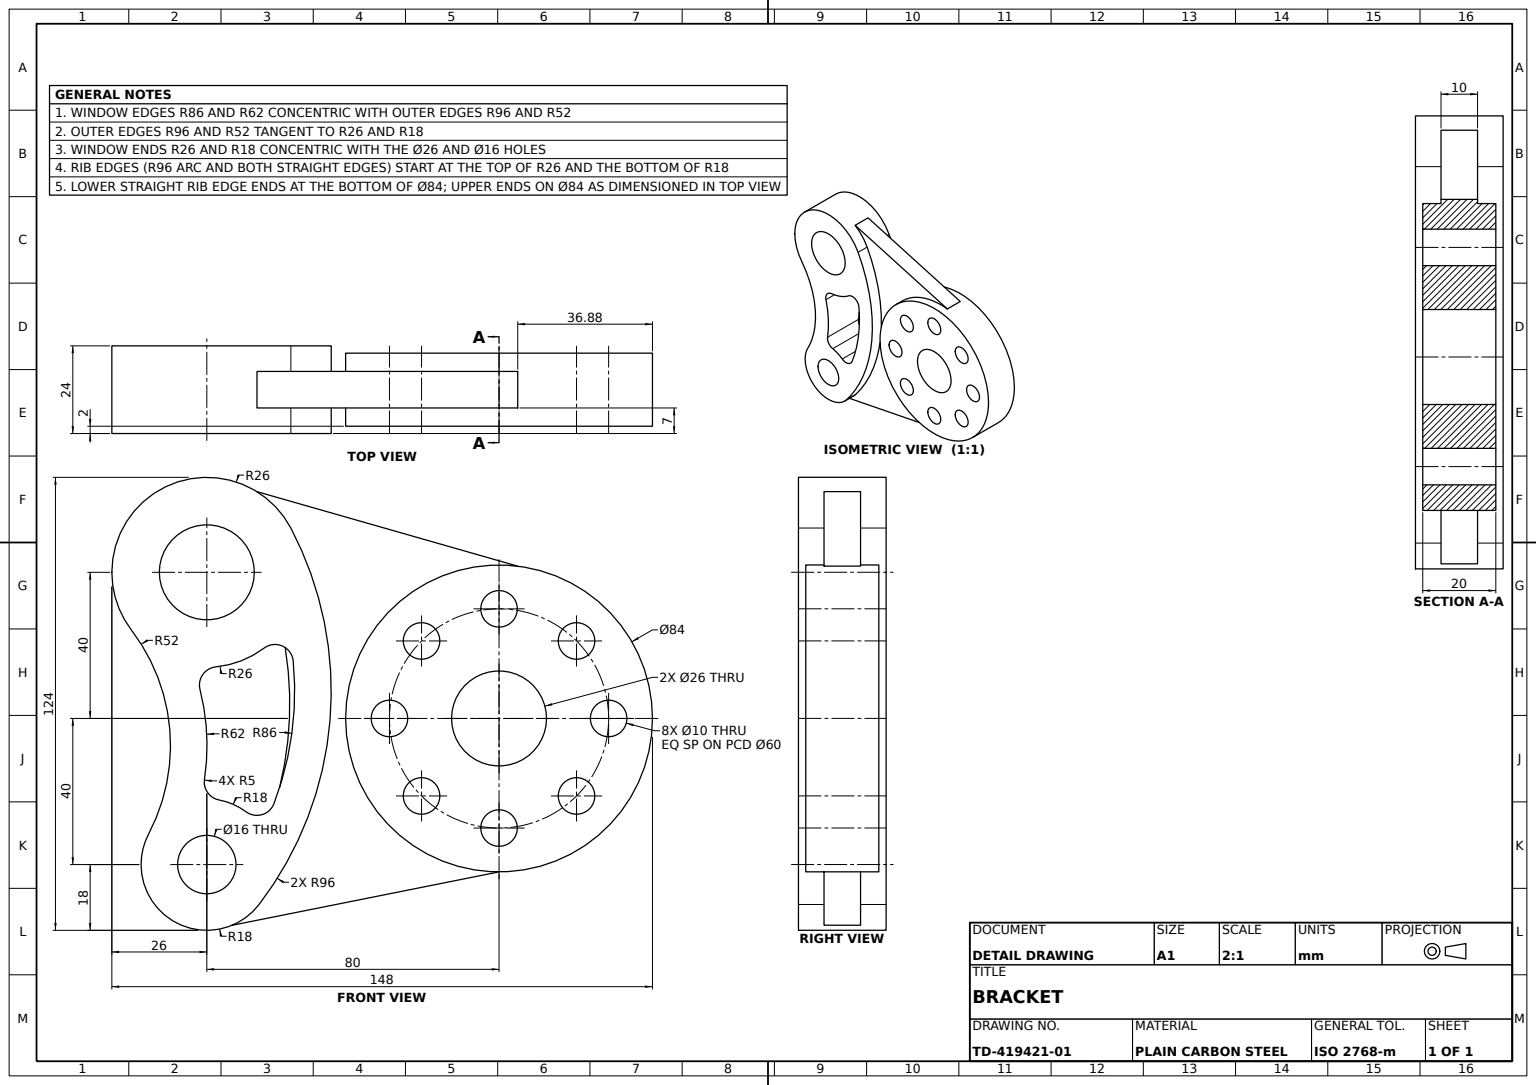
from build123d import *

# Parameters (mm, degrees)
LINK_PLATE_PROFILE_R      = 8
LINK_PLATE_PROFILE_R_2    = 13
LINK_PLATE_DEPTH          = 24
HUB_DISC_PROFILE_84_R     = 42
HUB_DISC_84_DEPTH         = 10
HUB_RIB_DEPTH             = 5
HUB_CENTRE_BORE_SKETCH_R  = 13
HUB_CENTRE_BORE_DEPTH     = 127.791166885
HUB_HOLE_SKETCH_R         = 5
HUB_HOLE_DEPTH            = 127.791166885
HUB_HOLE_PATTERN_8X_COUNT = 8


with BuildPart() as part:
    # Link Plate Profile → Link Plate (new body)
    with BuildSketch(Plane.XY):
        with BuildLine():
            ThreePointArc((-65.704893873, -50.938461538), (-46.286814024, -0.688477763), (-56.99168633, 52.108571429))
            ThreePointArc((-56.99168633, 52.108571429), (-94.004081038, 61.906293942), (-100.648486627, 24.2))
            ThreePointArc((-100.648486627, 24.2), (-90.130360042, -3.018741212), (-95.928832541, -31.617142857))
            ThreePointArc((-95.928832541, -31.617142857), (-89.695133026, -55.165895806), (-65.704893873, -50.938461538))
        make_face()
        with Locations((-80, -40)):
            Circle(LINK_PLATE_PROFILE_R, mode=Mode.SUBTRACT)
        with BuildLine():
            ThreePointArc((-81.86521747, 7.908967037), (-81.11107364, 12.018176986), (-77.500675884, 14.120406128))
            ThreePointArc((-77.500675884, 14.120406128), (-70.565087966, 15.772279618), (-64.338947731, 19.245929512))
            ThreePointArc((-64.338947731, 19.245929512), (-59.317592319, 19.833129635), (-56.350771542, 15.739623969))
            ThreePointArc((-56.350771542, 15.739623969), (-56.717251337, -4.095758702), (-61.619133807, -23.319396791))
            ThreePointArc((-61.619133807, -23.319396791), (-64.890999648, -26.333889771), (-69.26986273, -25.547866796))
            ThreePointArc((-69.26986273, -25.547866796), (-72.768447006, -23.516534306), (-76.632322996, -22.317840867))
            ThreePointArc((-76.632322996, -22.317840867), (-79.776843452, -20.296408854), (-80.640782737, -16.659403878))
            ThreePointArc((-80.640782737, -16.659403878), (-80.022314885, -4.313883718), (-81.86521747, 7.908967037))
        make_face(mode=Mode.SUBTRACT)
        with Locations((-80, 40)):
            Circle(LINK_PLATE_PROFILE_R_2, mode=Mode.SUBTRACT)
    extrude(amount=LINK_PLATE_DEPTH)



with BuildPart() as body_2:
    # Hub Disc Profile Ø84 → Hub Disc Ø84 (new, symmetric)
    with BuildSketch(Plane.XY.offset(12)):
        Circle(HUB_DISC_PROFILE_84_R)
    extrude(amount=HUB_DISC_84_DEPTH, both=True)


with BuildPart() as part_1:
    add(part.part)

    add(body_2.part)  # Hub Rib merges body 2
    # Rib Profile → Hub Rib (add, symmetric)
    with BuildSketch(Plane.XY.offset(12)):
        with BuildLine():
            Line((-80, 66), (5.116324571, 41.687206945))
            ThreePointArc((5.116324571, 41.687206945), (-41.921728803, 2.562938577), (0, -42))
            Line((0, -42), (-80, -58))
            ThreePointArc((-80, -58), (-57.293928807, 4), (-80, 66))
        make_face()
    extrude(amount=HUB_RIB_DEPTH, both=True)

    # Hub Centre Bore Sketch → Hub Centre Bore (cut, through all)
    with BuildSketch(Plane.XY.offset(22)):
        Circle(HUB_CENTRE_BORE_SKETCH_R)
    extrude(amount=-HUB_CENTRE_BORE_DEPTH, mode=Mode.SUBTRACT)

    # Hub Hole Sketch → Hub Hole (cut, through all)
    with BuildSketch(Plane.XY.offset(22)):
        with Locations((0, 30)):
            Circle(HUB_HOLE_SKETCH_R)
    hub_hole = extrude(amount=-HUB_HOLE_DEPTH, mode=Mode.SUBTRACT)

    # Hub Hole Pattern 8x: Hub Hole ×8 about axis
    hub_hole_pattern_8x_axis = Axis((0, 0, 0), (0, 0, 1))
    for i in range(1, HUB_HOLE_PATTERN_8X_COUNT):
        add(hub_hole.rotate(hub_hole_pattern_8x_axis, i * 360 / HUB_HOLE_PATTERN_8X_COUNT), mode=Mode.SUBTRACT)


solid = part_1.part
